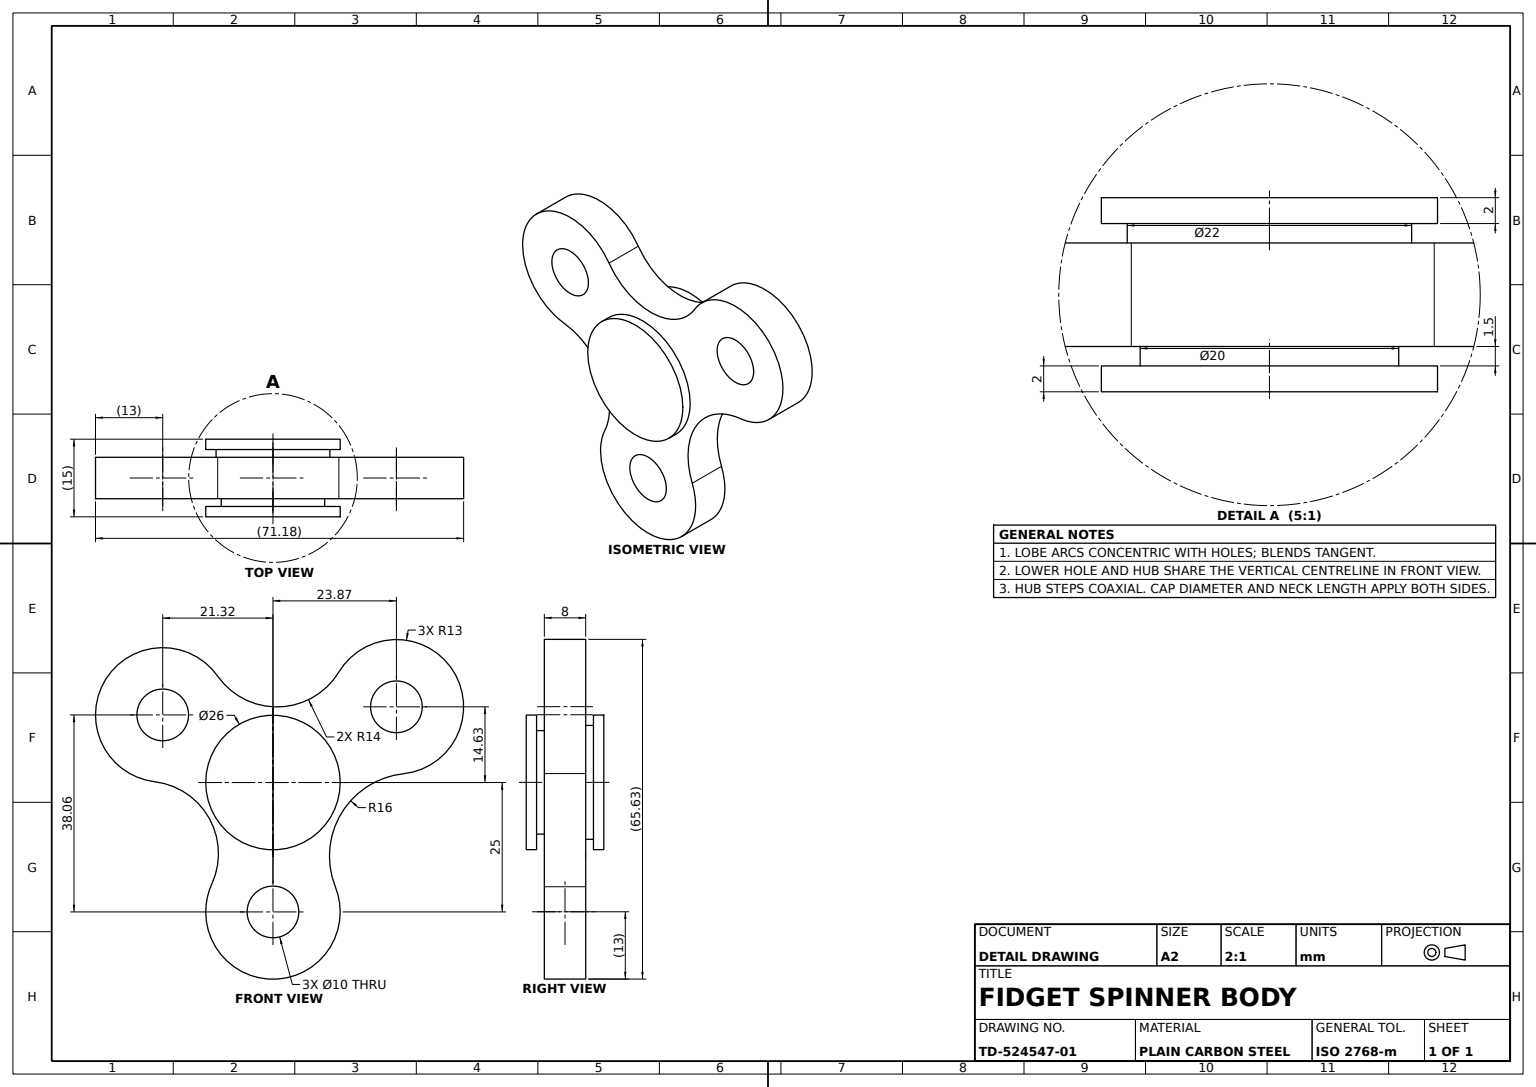
from build123d import *

# Parameters (mm, degrees)
SPINNER_BODY_DEPTH             = 8
HUB_BOSS_10_SKETCH_R           = 10
HUB_BOSS_10_DEPTH              = 1.5
HUB_BOSS_11_SKETCH_R           = 11
HUB_BOSS_11_DEPTH              = 1.5
HUB_CAP_13_ON_11_BOSS_SKETCH_R = 13
HUB_CAP_13_ON_11_BOSS_DEPTH    = 2
HUB_START                      = 2
HUB_CAP_13_ON_10_BOSS_SKETCH_R = 13
HUB_CAP_13_ON_10_BOSS_DEPTH    = 2
LOBE_HOLES_3X_10_SKETCH_R      = 10
LOBE_HOLES_3X_10_DEPTH         = 8
LOBE_RINGS_3X_10_9_SKETCH_R    = 10
LOBE_RINGS_3X_10_9_SKETCH_R_2  = 9
LOBE_RINGS_3X_10_9_DEPTH       = 8
LOBE_RINGS_3X_9_6_SKETCH_R     = 9
LOBE_RINGS_3X_9_6_SKETCH_R_2   = 6
LOBE_RINGS_3X_9_6_DEPTH        = 8
LOBE_RINGS_3X_6_5_SKETCH_R     = 6
LOBE_RINGS_3X_6_5_SKETCH_R_2   = 5
LOBE_RINGS_3X_6_5_DEPTH        = 8


with BuildPart() as part:
    # Spinner Body Sketch → Spinner Body (new body)
    with BuildSketch(Plane.XY):
        with BuildLine():
            ThreePointArc((-11.816475763, -19.580507354), (-0.317877053, -37.996113041), (12.067302022, -20.164690091))
            ThreePointArc((12.067302022, -20.164690091), (13.213407519, -5.958437932), (25.234931886, 1.697547316))
            ThreePointArc((25.234931886, 1.697547316), (34.838281601, 21.597841349), (12.74333417, 21.35427128))
            ThreePointArc((12.74333417, 21.35427128), (1.248689911, 14.609217628), (-10.684542323, 20.543909185))
            ThreePointArc((-10.684542323, 20.543909185), (-32.475062427, 19.731453355), (-22.869218634, 0.155585152))
            ThreePointArc((-22.869218634, 0.155585152), (-12.326967101, -6.903433276), (-11.816475763, -19.580507354))
        make_face()
    extrude(amount=SPINNER_BODY_DEPTH)

    # Hub Boss Ø10 Sketch → Hub Boss Ø10 (add)
    with BuildSketch(Plane.XY.offset(8)):
        Circle(HUB_BOSS_10_SKETCH_R)
    extrude(amount=HUB_BOSS_10_DEPTH)

    # Hub Boss Ø11 Sketch → Hub Boss Ø11 (add)
    with BuildSketch(Plane(origin=(0, 0, 0), x_dir=(-1, 0, 0), z_dir=(0, 0, -1))):
        with Locations(Location((0, 0, 0), (0, 0, 180))):
            Circle(HUB_BOSS_11_SKETCH_R)
    extrude(amount=HUB_BOSS_11_DEPTH)

    # Hub Cap Ø13 on Ø11 Boss Sketch → Hub Cap Ø13 on Ø11 Boss (add)
    with BuildSketch(Plane(origin=(0, 0, -1.5), x_dir=(-1, 0, 0), z_dir=(0, 0, -1))):
        Circle(HUB_CAP_13_ON_11_BOSS_SKETCH_R)
    extrude(amount=HUB_CAP_13_ON_11_BOSS_DEPTH)

    # Hub Cap Ø13 on Ø10 Boss Sketch → Hub Cap Ø13 on Ø10 Boss (add)
    with BuildSketch(Plane.XY.offset(9.5).offset(HUB_START)):
        with Locations(Location((0, 0, 0), (0, 0, 180))):
            Circle(HUB_CAP_13_ON_10_BOSS_SKETCH_R)
    extrude(amount=-HUB_CAP_13_ON_10_BOSS_DEPTH)

    # Lobe Holes 3xØ10 Sketch → Lobe Holes 3xØ10 (cut)
    with BuildSketch(Plane(origin=(0, 0, 0), x_dir=(-1, 0, 0), z_dir=(0, 0, -1))):
        with Locations((-23.866329129, 14.6253053)):
            Circle(LOBE_HOLES_3X_10_SKETCH_R)
        with Locations((21.316004109, 13.062464118)):
            Circle(LOBE_HOLES_3X_10_SKETCH_R)
        with Locations((0, -25)):
            Circle(LOBE_HOLES_3X_10_SKETCH_R)
    extrude(amount=-LOBE_HOLES_3X_10_DEPTH, mode=Mode.SUBTRACT)

    # Lobe Rings 3xØ10-Ø9 Sketch → Lobe Rings 3xØ10-Ø9 (add)
    # profile 1 of 3: a face of its own
    with BuildSketch(Plane(origin=(0, 0, 0), x_dir=(-1, 0, 0), z_dir=(0, 0, -1))):
        with Locations((-23.866329129, 14.6253053)):
            Circle(LOBE_RINGS_3X_10_9_SKETCH_R)
        with Locations((-23.866329129, 14.6253053)):
            Circle(LOBE_RINGS_3X_10_9_SKETCH_R_2, mode=Mode.SUBTRACT)
    # profile 2 of 3: a face of its own
    with BuildSketch(Plane(origin=(0, 0, 0), x_dir=(-1, 0, 0), z_dir=(0, 0, -1))):
        with Locations((21.316004109, 13.062464118)):
            Circle(LOBE_RINGS_3X_10_9_SKETCH_R)
        with Locations((21.316004109, 13.062464118)):
            Circle(LOBE_RINGS_3X_10_9_SKETCH_R_2, mode=Mode.SUBTRACT)
    # profile 3 of 3: a face of its own
    with BuildSketch(Plane(origin=(0, 0, 0), x_dir=(-1, 0, 0), z_dir=(0, 0, -1))):
        with Locations((0, -25)):
            Circle(LOBE_RINGS_3X_10_9_SKETCH_R)
        with Locations((0, -25)):
            Circle(LOBE_RINGS_3X_10_9_SKETCH_R_2, mode=Mode.SUBTRACT)
    extrude(amount=-LOBE_RINGS_3X_10_9_DEPTH)

    # Lobe Rings 3xØ9-Ø6 Sketch → Lobe Rings 3xØ9-Ø6 (add)
    # profile 1 of 3: a face of its own
    with BuildSketch(Plane(origin=(0, 0, 0), x_dir=(-1, 0, 0), z_dir=(0, 0, -1))):
        with Locations((-23.866329129, 14.6253053)):
            Circle(LOBE_RINGS_3X_9_6_SKETCH_R)
        with Locations((-23.866329129, 14.6253053)):
            Circle(LOBE_RINGS_3X_9_6_SKETCH_R_2, mode=Mode.SUBTRACT)
    # profile 2 of 3: a face of its own
    with BuildSketch(Plane(origin=(0, 0, 0), x_dir=(-1, 0, 0), z_dir=(0, 0, -1))):
        with Locations((21.316004109, 13.062464118)):
            Circle(LOBE_RINGS_3X_9_6_SKETCH_R)
        with Locations((21.316004109, 13.062464118)):
            Circle(LOBE_RINGS_3X_9_6_SKETCH_R_2, mode=Mode.SUBTRACT)
    # profile 3 of 3: a face of its own
    with BuildSketch(Plane(origin=(0, 0, 0), x_dir=(-1, 0, 0), z_dir=(0, 0, -1))):
        with Locations((0, -25)):
            Circle(LOBE_RINGS_3X_9_6_SKETCH_R)
        with Locations((0, -25)):
            Circle(LOBE_RINGS_3X_9_6_SKETCH_R_2, mode=Mode.SUBTRACT)
    extrude(amount=-LOBE_RINGS_3X_9_6_DEPTH)

    # Lobe Rings 3xØ6-Ø5 Sketch → Lobe Rings 3xØ6-Ø5 (add)
    # profile 1 of 3: a face of its own
    with BuildSketch(Plane(origin=(0, 0, 0), x_dir=(-1, 0, 0), z_dir=(0, 0, -1))):
        with Locations((-23.866329129, 14.6253053)):
            Circle(LOBE_RINGS_3X_6_5_SKETCH_R)
        with Locations((-23.866329129, 14.6253053)):
            Circle(LOBE_RINGS_3X_6_5_SKETCH_R_2, mode=Mode.SUBTRACT)
    # profile 2 of 3: a face of its own
    with BuildSketch(Plane(origin=(0, 0, 0), x_dir=(-1, 0, 0), z_dir=(0, 0, -1))):
        with Locations((21.316004109, 13.062464118)):
            Circle(LOBE_RINGS_3X_6_5_SKETCH_R)
        with Locations((21.316004109, 13.062464118)):
            Circle(LOBE_RINGS_3X_6_5_SKETCH_R_2, mode=Mode.SUBTRACT)
    # profile 3 of 3: a face of its own
    with BuildSketch(Plane(origin=(0, 0, 0), x_dir=(-1, 0, 0), z_dir=(0, 0, -1))):
        with Locations((0, -25)):
            Circle(LOBE_RINGS_3X_6_5_SKETCH_R)
        with Locations((0, -25)):
            Circle(LOBE_RINGS_3X_6_5_SKETCH_R_2, mode=Mode.SUBTRACT)
    extrude(amount=-LOBE_RINGS_3X_6_5_DEPTH)


solid = part.part
